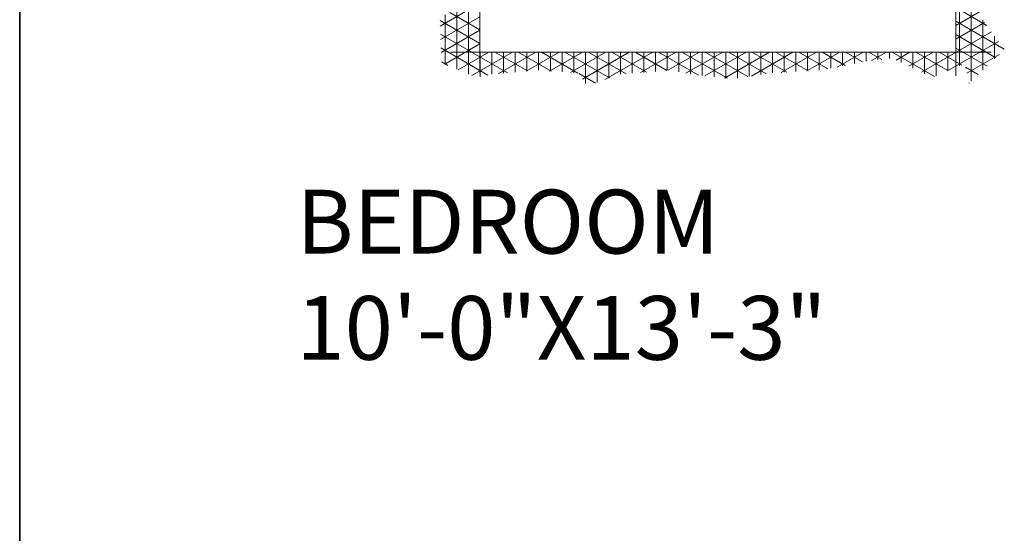
# Model space of a CAD drawing. Units: inches. Extents: x 3731 to 4318, y 1310 to 2388.
# Tile 25 of 57: x 3840 to 3948, y 1787 to 1844. Entities that reach past the tile are written whole.
import ezdxf

# ---------------------------------------------------------------- set-up
doc = ezdxf.new("R2010")
doc.units = ezdxf.units.IN
for name, color, linetype, lineweight in [('A-AREA-IDEN', 7, 'Continuous', 18), ('A-FURN', 8, 'Continuous', 13), ('A-WALL', 7, 'Continuous', 35)]:
    doc.layers.add(name, color=color, linetype=linetype, lineweight=lineweight)
doc.styles.get("Standard").update_dxf_attribs({"font": 'arial.ttf'})

# ---------------------------------------------------------------- blocks, each defined once
blk = doc.blocks.new('A$C200C7901')
for p, q in [((2.3121, 1.6596), (2.3121, 0.0201)), ((1.0407, 0.0275), (1.0407, 0.4323)), ((2.4073, 0.0839), (0.9625, 0.0839))]:
    blk.add_line(p, q)
at = {"linetype": 'ByBlock'}
for p, q in [((2.3224, 0.0468), (2.3224, 1.6627)), ((2.3224, 0.0468), (2.3224, 1.6627)), ((2.3537, 0.0056), (2.3537, 1.634)), ((2.3537, 0.0056), (2.3537, 1.634)), ((0.9344, 0.153), (1.0407, 0.2144)), ((0.9344, 0.153), (1.0407, 0.2144)), ((1.0099, 0.0251), (1.0099, 0.2117)), ((1.0099, 0.0251), (1.0099, 0.2117)), ((0.9602, 0.1893), (1.0407, 0.1428)), ((0.9602, 0.1893), (1.0407, 0.1428)), ((0.9787, 0.0381), (0.9787, 0.1976)), ((0.9787, 0.0381), (0.9787, 0.1976)), ((2.3121, 0.2026), (2.3953, 0.1545)), ((2.3121, 0.2026), (2.3953, 0.1545)), ((2.3121, 0.1546), (2.3755, 0.1912)), ((2.3121, 0.1546), (2.3755, 0.1912)), ((0.9339, 0.1684), (1.0407, 0.1067)), ((0.9339, 0.1684), (1.0407, 0.1067)), ((0.9355, 0.1176), (1.0407, 0.1783)), ((0.9355, 0.1176), (1.0407, 0.1783)), ((0.9474, 0.0512), (0.9474, 0.1835)), ((0.9474, 0.0512), (0.9474, 0.1835)), ((2.3121, 0.1665), (2.4419, 0.0916)), ((2.3121, 0.1665), (2.4419, 0.0916)), ((2.3121, 0.1185), (2.3891, 0.163)), ((2.3121, 0.1185), (2.3891, 0.163)), ((2.3849, 0.0355), (2.3849, 0.1686)), ((2.3849, 0.0355), (2.3849, 0.1686)), ((0.935, 0.1316), (1.114, 0.0283)), ((0.935, 0.1316), (1.114, 0.0283)), ((0.9366, 0.0822), (1.0407, 0.1422)), ((0.9366, 0.0822), (1.0407, 0.1422)), ((2.2208, 0.0297), (2.4078, 0.1377)), ((2.2208, 0.0297), (2.4078, 0.1377)), ((0.9463, 0.0516), (1.0407, 0.1061)), ((0.9463, 0.0516), (1.0407, 0.1061)), ((2.2903, 0.0337), (2.4265, 0.1124)), ((2.2903, 0.0337), (2.4265, 0.1124)), ((2.3121, 0.1304), (2.4193, 0.0685)), ((2.3121, 0.1304), (2.4193, 0.0685)), ((2.4162, 0.0655), (2.4162, 0.1264)), ((2.4162, 0.0655), (2.4162, 0.1264)), ((0.9362, 0.0948), (1.0616, 0.0225)), ((0.9362, 0.0948), (1.0616, 0.0225)), ((0.9826, 0.0365), (1.0647, 0.0839)), ((0.9826, 0.0365), (1.0647, 0.0839)), ((1.0189, 0.0214), (1.1272, 0.0839)), ((1.0189, 0.0214), (1.1272, 0.0839)), ((1.0412, 0.0179), (1.0412, 0.0839)), ((1.0412, 0.0179), (1.0412, 0.0839)), ((1.0724, 0.0243), (1.0724, 0.0839)), ((1.0724, 0.0243), (1.0724, 0.0839)), ((1.0801, 0.0839), (1.1675, 0.0335)), ((1.0801, 0.0839), (1.1675, 0.0335)), ((1.0891, 0.0259), (1.1897, 0.0839)), ((1.0891, 0.0259), (1.1897, 0.0839)), ((1.1037, 0.0273), (1.1037, 0.0839)), ((1.1037, 0.0273), (1.1037, 0.0839)), ((1.1349, 0.0303), (1.1349, 0.0839)), ((1.1349, 0.0303), (1.1349, 0.0839)), ((1.1426, 0.0839), (1.2313, 0.0327)), ((1.1426, 0.0839), (1.2313, 0.0327)), ((1.1642, 0.0331), (1.2522, 0.0839)), ((1.1642, 0.0331), (1.2522, 0.0839)), ((1.1662, 0.0333), (1.1662, 0.0839)), ((1.1662, 0.0333), (1.1662, 0.0839)), ((1.1974, 0.0351), (1.1974, 0.0839)), ((1.1974, 0.0351), (1.1974, 0.0839)), ((1.2051, 0.0839), (1.3023, 0.0278)), ((1.2051, 0.0839), (1.3023, 0.0278)), ((1.2266, 0.033), (1.3147, 0.0839)), ((1.2266, 0.033), (1.3147, 0.0839)), ((1.2287, 0.0329), (1.2287, 0.0839)), ((1.2287, 0.0329), (1.2287, 0.0839)), ((1.2599, 0.0308), (1.2599, 0.0839)), ((1.2599, 0.0308), (1.2599, 0.0839)), ((1.2676, 0.0839), (1.3871, 0.015)), ((1.2676, 0.0839), (1.3871, 0.015)), ((1.2824, 0.0292), (1.3772, 0.0839)), ((1.2824, 0.0292), (1.3772, 0.0839)), ((1.2912, 0.0286), (1.2912, 0.0839)), ((1.2912, 0.0286), (1.2912, 0.0839)), ((1.3146, 0.0117), (1.4397, 0.0839)), ((1.3146, 0.0117), (1.4397, 0.0839)), ((1.3224, 0), (1.3224, 0.0839)), ((1.3224, 0), (1.3224, 0.0839)), ((1.3301, 0.0839), (1.4312, 0.0256)), ((1.3301, 0.0839), (1.4312, 0.0256)), ((1.3537, 0.0022), (1.3537, 0.0839)), ((1.3537, 0.0022), (1.3537, 0.0839)), ((1.3743, 0.0101), (1.5022, 0.0839)), ((1.3743, 0.0101), (1.5022, 0.0839)), ((1.3849, 0.0141), (1.3849, 0.0839)), ((1.3849, 0.0141), (1.3849, 0.0839)), ((1.3926, 0.0839), (1.4856, 0.0302)), ((1.3926, 0.0839), (1.4856, 0.0302)), ((1.4162, 0.0243), (1.4162, 0.0839)), ((1.4162, 0.0243), (1.4162, 0.0839)), ((1.4474, 0.027), (1.4474, 0.0839)), ((1.4474, 0.027), (1.4474, 0.0839)), ((1.4551, 0.0839), (1.54, 0.0349)), ((1.4551, 0.0839), (1.54, 0.0349)), ((1.4693, 0.0288), (1.5647, 0.0839)), ((1.4693, 0.0288), (1.5647, 0.0839)), ((1.4787, 0.0296), (1.4787, 0.0839)), ((1.4787, 0.0296), (1.4787, 0.0839)), ((1.5099, 0.0323), (1.5099, 0.0839)), ((1.5099, 0.0323), (1.5099, 0.0839)), ((1.5176, 0.0839), (1.6251, 0.0219)), ((1.5176, 0.0839), (1.6251, 0.0219)), ((1.5412, 0.035), (1.5412, 0.0839)), ((1.5412, 0.035), (1.5412, 0.0839)), ((1.5427, 0.0351), (1.6272, 0.0839)), ((1.5427, 0.0351), (1.6272, 0.0839)), ((1.5724, 0.0308), (1.5724, 0.0839)), ((1.5724, 0.0308), (1.5724, 0.0839)), ((1.5801, 0.0839), (1.7018, 0.0137)), ((1.5801, 0.0839), (1.7018, 0.0137)), ((1.5911, 0.027), (1.6897, 0.0839)), ((1.5911, 0.027), (1.6897, 0.0839)), ((1.6037, 0.0245), (1.6037, 0.0839)), ((1.6037, 0.0245), (1.6037, 0.0839)), ((1.6349, 0.0208), (1.6349, 0.0839)), ((1.6349, 0.0208), (1.6349, 0.0839)), ((1.6416, 0.0201), (1.7522, 0.0839)), ((1.6416, 0.0201), (1.7522, 0.0839)), ((1.6426, 0.0839), (1.7565, 0.0182)), ((1.6426, 0.0839), (1.7565, 0.0182)), ((1.6662, 0.0175), (1.6662, 0.0839)), ((1.6662, 0.0175), (1.6662, 0.0839)), ((1.6944, 0.0145), (1.8147, 0.0839)), ((1.6944, 0.0145), (1.8147, 0.0839)), ((1.6974, 0.0141), (1.6974, 0.0839)), ((1.6974, 0.0141), (1.6974, 0.0839)), ((1.7051, 0.0839), (1.8054, 0.026)), ((1.7051, 0.0839), (1.8054, 0.026)), ((1.7287, 0.0137), (1.7287, 0.0839)), ((1.7287, 0.0137), (1.7287, 0.0839)), ((1.7599, 0.0187), (1.7599, 0.0839)), ((1.7599, 0.0187), (1.7599, 0.0839)), ((1.7659, 0.0197), (1.8772, 0.0839)), ((1.7659, 0.0197), (1.8772, 0.0839)), ((1.7676, 0.0839), (1.8606, 0.0303)), ((1.7676, 0.0839), (1.8606, 0.0303)), ((1.7912, 0.0237), (1.7912, 0.0839)), ((1.7912, 0.0237), (1.7912, 0.0839)), ((1.8224, 0.0281), (1.8224, 0.0839)), ((1.8224, 0.0281), (1.8224, 0.0839)), ((1.8301, 0.0839), (1.9175, 0.0335)), ((1.8301, 0.0839), (1.9175, 0.0335)), ((1.8452, 0.0294), (1.9397, 0.0839)), ((1.8452, 0.0294), (1.9397, 0.0839)), ((1.8537, 0.0299), (1.8537, 0.0839)), ((1.8537, 0.0299), (1.8537, 0.0839)), ((1.8849, 0.0316), (1.8849, 0.0839)), ((1.8849, 0.0316), (1.8849, 0.0839)), ((1.8926, 0.0839), (1.9706, 0.0389)), ((1.8926, 0.0839), (1.9706, 0.0389)), ((1.9146, 0.0333), (2.0022, 0.0839)), ((1.9146, 0.0333), (2.0022, 0.0839)), ((1.9162, 0.0334), (1.9162, 0.0839)), ((1.9162, 0.0334), (1.9162, 0.0839)), ((1.9474, 0.0352), (1.9474, 0.0839)), ((1.9474, 0.0352), (1.9474, 0.0839)), ((1.9551, 0.0839), (2.017, 0.0482)), ((1.9551, 0.0839), (2.017, 0.0482)), ((1.9787, 0.0405), (1.9787, 0.0839)), ((1.9787, 0.0405), (1.9787, 0.0839)), ((1.9953, 0.0438), (2.0647, 0.0839)), ((1.9953, 0.0438), (2.0647, 0.0839)), ((2.0099, 0.0468), (2.0099, 0.0839)), ((2.0099, 0.0468), (2.0099, 0.0839)), ((2.0176, 0.0839), (2.0634, 0.0575)), ((2.0176, 0.0839), (2.0634, 0.0575)), ((2.0412, 0.053), (2.0412, 0.0839)), ((2.0412, 0.053), (2.0412, 0.0839)), ((2.0724, 0.0592), (2.0724, 0.0839)), ((2.0724, 0.0592), (2.0724, 0.0839)), ((2.0801, 0.0839), (2.1147, 0.0639)), ((2.0801, 0.0839), (2.1147, 0.0639)), ((2.0873, 0.0609), (2.1272, 0.0839)), ((2.0873, 0.0609), (2.1272, 0.0839)), ((2.1037, 0.0627), (2.1037, 0.0839)), ((2.1037, 0.0627), (2.1037, 0.0839)), ((2.1349, 0.0662), (2.1349, 0.0839)), ((2.1349, 0.0662), (2.1349, 0.0839)), ((2.1426, 0.0839), (2.2557, 0.0186)), ((2.1426, 0.0839), (2.2557, 0.0186)), ((2.1526, 0.0625), (2.1897, 0.0839)), ((2.1526, 0.0625), (2.1897, 0.0839)), ((2.1662, 0.056), (2.1662, 0.0839)), ((2.1662, 0.056), (2.1662, 0.0839)), ((2.1867, 0.0461), (2.2522, 0.0839)), ((2.1867, 0.0461), (2.2522, 0.0839)), ((2.1974, 0.041), (2.1974, 0.0839)), ((2.1974, 0.041), (2.1974, 0.0839)), ((2.2051, 0.0839), (2.2913, 0.0342)), ((2.2051, 0.0839), (2.2913, 0.0342)), ((2.2287, 0.0259), (2.2287, 0.0839)), ((2.2287, 0.0259), (2.2287, 0.0839)), ((2.2599, 0.0205), (2.2599, 0.0839)), ((2.2599, 0.0205), (2.2599, 0.0839)), ((2.2676, 0.0839), (2.3285, 0.0488)), ((2.2676, 0.0839), (2.3285, 0.0488)), ((2.2912, 0.0341), (2.2912, 0.0839)), ((2.2912, 0.0341), (2.2912, 0.0839)), ((2.3121, 0.0943), (2.3958, 0.046)), ((2.3121, 0.0943), (2.3958, 0.046)), ((0.9374, 0.0581), (0.9545, 0.0482)), ((0.9374, 0.0581), (0.9545, 0.0482)), ((2.3417, 0.0273), (2.429, 0.0777)), ((2.3417, 0.0273), (2.429, 0.0777)), ((1.3048, 0.0264), (1.3494, 0.0006)), ((1.3048, 0.0264), (1.3494, 0.0006)), ((2.338, 0.0433), (2.3723, 0.0235)), ((2.338, 0.0433), (2.3723, 0.0235)), ((2.3476, 0.0017), (2.3488, 0.001)), ((2.3476, 0.0017), (2.3488, 0.001))]:
    blk.add_line(p, q, dxfattribs=at)

msp = doc.modelspace()

# ---------------------------------------------------------------- linework, layer by layer
at = {"layer": 'A-WALL'}
msp.add_line((3840.21, 1938.38), (3840.21, 1779.38), dxfattribs=at)

# ---------------------------------------------------------------- block references
at = {"layer": 'A-FURN', "xscale": 41.1071563136412, "yscale": 41.1071563136412, "zscale": 41.1071563136412}
msp.add_blockref('A$C200C7901', (3848, 1836.63), dxfattribs=at)

# ---------------------------------------------------------------- texts
at = {"layer": 'A-AREA-IDEN', "insert": (3870.61, 1824.95), "char_height": 7, "attachment_point": 1}
msp.add_mtext_dynamic_manual_height_columns('BEDROOM\\P10\'-0"X13\'-3"', width=47.0437, gutter_width=12.5, heights=[0], dxfattribs=at)

doc.saveas('drawing.dxf')
